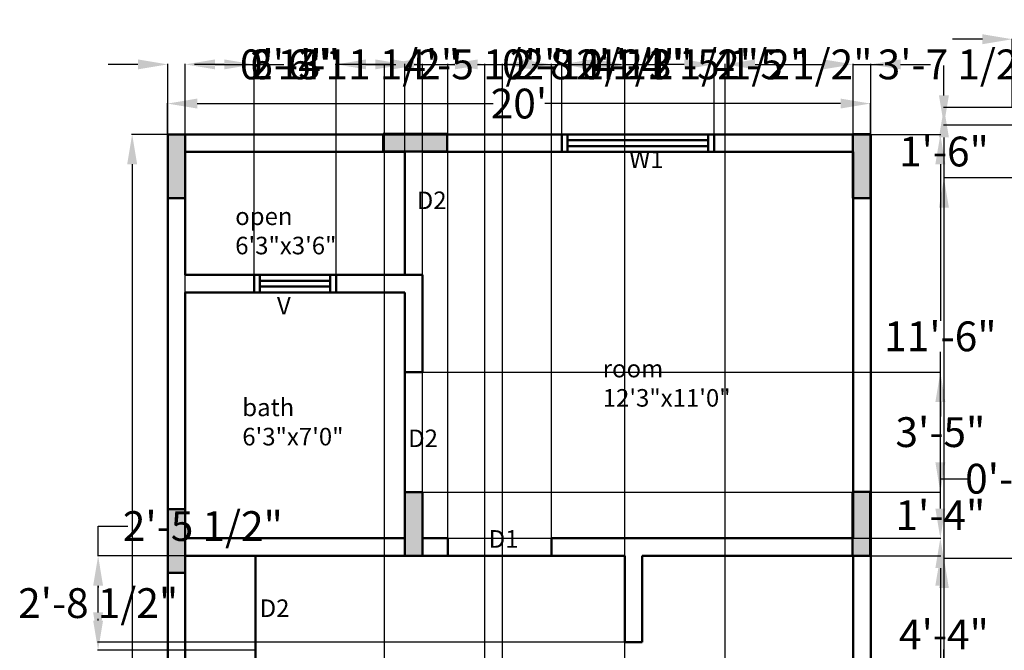
# Model space of a CAD drawing. Units: inches. Extents: x 21 to 3450, y 4 to 2137.
# Tile 2 of 14: x 2177 to 2513, y 1321 to 1537. Entities that reach past the tile are written whole.
import ezdxf

# ---------------------------------------------------------------- set-up
doc = ezdxf.new("R2010")
doc.units = ezdxf.units.IN
doc.header["$MEASUREMENT"] = 0
for name, color, linetype, lineweight in [('A-ANNO-DIMS', 2, 'Continuous', 18), ('A-ANNO-TEXT', 7, 'Continuous', 18), ('A-AREA-IDEN', 3, 'Continuous', 18), ('A-WALL', 7, 'Continuous', 50), ('A-WALL-PATT', 8, 'Continuous', 13)]:
    doc.layers.add(name, color=color, linetype=linetype, lineweight=lineweight)
doc.styles.get("Standard").update_dxf_attribs({"font": 'arial.ttf'})
doc.dimstyles.get("Standard").update_dxf_attribs({"dimtxt": 10.18, "dimasz": 10.18, "dimexe": 0.18, "dimexo": 0.0625, "dimgap": 0.09, "dimtad": 0, "dimtih": 1, "dimtoh": 1, "dimdec": 0, "dimzin": 0, "dimdsep": 46, "dimlunit": 3, "dimtxsty": 'Standard', "dimcen": 0.09, "dimadec": 0, "dimazin": 0, "dimtfac": 1, "dimtdec": 0, "dimtofl": 0, "dimtmove": 0, "dimatfit": 3, "dimfxl": 1, "dimtolj": 1, "dimtzin": 0, "dimarcsym": 0})

# ---------------------------------------------------------------- blocks, each defined once
blk = doc.blocks.new('*D1')
at = {"layer": 'A-ANNO-DIMS', "color": 0, "lineweight": -2, "transparency": 16777216}
for p, q in [((2227.33, 1497.5), (2215.09, 1497.5)), ((2215.27, 1487.32), (2215.27, 1292.79)), ((2215.27, 1087.68), (2215.27, 1282.21)), ((2227.33, 1077.5), (2215.09, 1077.5))]:
    blk.add_line(p, q, dxfattribs=at)
at = {"layer": 'A-ANNO-DIMS', "color": 0, "transparency": 16777216}
for points in [[(2213.57, 1487.32), (2216.97, 1487.32), (2215.27, 1497.5)], [(2213.57, 1087.68), (2216.97, 1087.68), (2215.27, 1077.5)]]:
    blk.add_solid(points, dxfattribs=at)
at = {"layer": 'Defpoints', "color": 0, "transparency": 16777216}
for p in [(2227.4, 1497.5), (2215.27, 1077.5), (2227.4, 1077.5)]:
    blk.add_point(p, dxfattribs=at)
at = {"layer": 'A-ANNO-DIMS', "color": 0, "transparency": 16777216, "insert": (2215.27, 1287.5), "char_height": 10.18, "attachment_point": 5}
blk.add_mtext("\\A1;35'", dxfattribs=at)
blk = doc.blocks.new('*D2')
at = {"layer": 'A-ANNO-DIMS', "color": 0, "lineweight": -2, "transparency": 16777216}
for p, q in [((2227.33, 1497.56), (2227.33, 1508.21)), ((2237.51, 1508.03), (2338.48, 1508.03)), ((2457.08, 1508.03), (2356.11, 1508.03)), ((2467.26, 1497.56), (2467.26, 1508.21))]:
    blk.add_line(p, q, dxfattribs=at)
at = {"layer": 'A-ANNO-DIMS', "color": 0, "transparency": 16777216}
for points in [[(2237.51, 1509.73), (2237.51, 1506.33), (2227.33, 1508.03)], [(2457.08, 1509.73), (2457.08, 1506.33), (2467.26, 1508.03)]]:
    blk.add_solid(points, dxfattribs=at)
at = {"layer": 'Defpoints', "color": 0, "transparency": 16777216}
for p in [(2467.26, 1508.03), (2227.33, 1497.5), (2467.26, 1497.5)]:
    blk.add_point(p, dxfattribs=at)
at = {"layer": 'A-ANNO-DIMS', "color": 0, "transparency": 16777216, "insert": (2347.3, 1508.03), "char_height": 10.18, "attachment_point": 5}
blk.add_mtext("\\A1;20'", dxfattribs=at)
blk = doc.blocks.new('*D34')
at = {"layer": 'A-ANNO-DIMS', "color": 0, "lineweight": -2, "transparency": 16777216}
for p, q in [((2217.22, 1521.41), (2207.04, 1521.41)), ((2227.4, 1497.56), (2227.4, 1521.59)), ((2233.4, 1491.56), (2233.4, 1521.59)), ((2243.58, 1521.41), (2253.76, 1521.41))]:
    blk.add_line(p, q, dxfattribs=at)
at = {"layer": 'A-ANNO-DIMS', "color": 0, "transparency": 16777216}
for points in [[(2217.22, 1523.11), (2217.22, 1519.72), (2227.4, 1521.41)], [(2243.58, 1523.11), (2243.58, 1519.72), (2233.4, 1521.41)]]:
    blk.add_solid(points, dxfattribs=at)
at = {"layer": 'Defpoints', "color": 0, "transparency": 16777216}
for p in [(2233.4, 1521.41), (2227.4, 1497.5), (2233.4, 1491.5)]:
    blk.add_point(p, dxfattribs=at)
at = {"layer": 'A-ANNO-DIMS', "color": 0, "transparency": 16777216, "insert": (2267.38, 1521.41), "char_height": 10.18, "attachment_point": 5}
blk.add_mtext('\\A1;0\'-6"', dxfattribs=at)
blk = doc.blocks.new('*D35')
at = {"layer": 'A-ANNO-DIMS', "color": 0, "lineweight": -2, "transparency": 16777216}
for p, q in [((2233.4, 1491.56), (2233.4, 1521.59)), ((2243.58, 1521.41), (2257.25, 1521.41)), ((2298.22, 1521.41), (2284.54, 1521.41)), ((2308.4, 1491.56), (2308.4, 1521.59))]:
    blk.add_line(p, q, dxfattribs=at)
at = {"layer": 'A-ANNO-DIMS', "color": 0, "transparency": 16777216}
for points in [[(2243.58, 1523.11), (2243.58, 1519.72), (2233.4, 1521.41)], [(2298.22, 1523.11), (2298.22, 1519.72), (2308.4, 1521.41)]]:
    blk.add_solid(points, dxfattribs=at)
at = {"layer": 'Defpoints', "color": 0, "transparency": 16777216}
for p in [(2308.4, 1521.41), (2233.4, 1491.5), (2308.4, 1491.5)]:
    blk.add_point(p, dxfattribs=at)
at = {"layer": 'A-ANNO-DIMS', "color": 0, "transparency": 16777216, "insert": (2270.9, 1521.41), "char_height": 10.18, "attachment_point": 5}
blk.add_mtext('\\A1;6\'-3"', dxfattribs=at)
blk = doc.blocks.new('*D36')
at = {"layer": 'A-ANNO-DIMS', "color": 0, "lineweight": -2, "transparency": 16777216}
for p, q in [((2298.22, 1521.41), (2288.04, 1521.41)), ((2308.4, 1491.56), (2308.4, 1521.59)), ((2361.9, 1497.56), (2361.9, 1521.59)), ((2372.08, 1521.41), (2382.26, 1521.41))]:
    blk.add_line(p, q, dxfattribs=at)
at = {"layer": 'A-ANNO-DIMS', "color": 0, "transparency": 16777216}
for points in [[(2298.22, 1523.11), (2298.22, 1519.72), (2308.4, 1521.41)], [(2372.08, 1523.11), (2372.08, 1519.72), (2361.9, 1521.41)]]:
    blk.add_solid(points, dxfattribs=at)
at = {"layer": 'Defpoints', "color": 0, "transparency": 16777216}
for p in [(2361.9, 1521.41), (2361.9, 1497.5), (2308.4, 1491.5)]:
    blk.add_point(p, dxfattribs=at)
at = {"layer": 'A-ANNO-DIMS', "color": 0, "transparency": 16777216, "insert": (2335.15, 1521.41), "char_height": 10.18, "attachment_point": 5}
blk.add_mtext('\\A1;4\'-5 1/2"', dxfattribs=at)
blk = doc.blocks.new('*D37')
at = {"layer": 'A-ANNO-DIMS', "color": 0, "lineweight": -2, "transparency": 16777216}
for p, q in [((2361.9, 1497.56), (2361.9, 1521.59)), ((2372.08, 1521.41), (2374.07, 1521.41)), ((2403.72, 1521.41), (2401.72, 1521.41)), ((2413.9, 1497.56), (2413.9, 1521.59))]:
    blk.add_line(p, q, dxfattribs=at)
at = {"layer": 'A-ANNO-DIMS', "color": 0, "transparency": 16777216}
for points in [[(2372.08, 1523.11), (2372.08, 1519.72), (2361.9, 1521.41)], [(2403.72, 1523.11), (2403.72, 1519.72), (2413.9, 1521.41)]]:
    blk.add_solid(points, dxfattribs=at)
at = {"layer": 'Defpoints', "color": 0, "transparency": 16777216}
for p in [(2413.9, 1521.41), (2361.9, 1497.5), (2413.9, 1497.5)]:
    blk.add_point(p, dxfattribs=at)
at = {"layer": 'A-ANNO-DIMS', "color": 0, "transparency": 16777216, "insert": (2387.9, 1521.41), "char_height": 10.18, "attachment_point": 5}
blk.add_mtext('\\A1;4\'-4"', dxfattribs=at)
blk = doc.blocks.new('*D38')
at = {"layer": 'A-ANNO-DIMS', "color": 0, "lineweight": -2, "transparency": 16777216}
for p, q in [((2403.72, 1521.41), (2393.54, 1521.41)), ((2413.9, 1497.56), (2413.9, 1521.59)), ((2467.4, 1497.56), (2467.4, 1521.59)), ((2477.58, 1521.41), (2487.76, 1521.41))]:
    blk.add_line(p, q, dxfattribs=at)
at = {"layer": 'A-ANNO-DIMS', "color": 0, "transparency": 16777216}
for points in [[(2403.72, 1523.11), (2403.72, 1519.72), (2413.9, 1521.41)], [(2477.58, 1523.11), (2477.58, 1519.72), (2467.4, 1521.41)]]:
    blk.add_solid(points, dxfattribs=at)
at = {"layer": 'Defpoints', "color": 0, "transparency": 16777216}
for p in [(2467.4, 1521.41), (2413.9, 1497.5), (2467.4, 1497.5)]:
    blk.add_point(p, dxfattribs=at)
at = {"layer": 'A-ANNO-DIMS', "color": 0, "transparency": 16777216, "insert": (2440.65, 1521.41), "char_height": 10.18, "attachment_point": 5}
blk.add_mtext('\\A1;4\'-5 1/2"', dxfattribs=at)
blk = doc.blocks.new('*D47')
at = {"layer": 'A-ANNO-DIMS', "color": 0, "lineweight": -2, "transparency": 16777216}
for p, q in [((2461.25, 1353.55), (2491.33, 1353.55)), ((2491.15, 1343.37), (2491.15, 1298.81)), ((2491.15, 1243.68), (2491.15, 1288.24)), ((2461.46, 1233.5), (2491.33, 1233.5))]:
    blk.add_line(p, q, dxfattribs=at)
at = {"layer": 'A-ANNO-DIMS', "color": 0, "transparency": 16777216}
for points in [[(2489.45, 1343.37), (2492.84, 1343.37), (2491.15, 1353.55)], [(2489.45, 1243.68), (2492.84, 1243.68), (2491.15, 1233.5)]]:
    blk.add_solid(points, dxfattribs=at)
at = {"layer": 'Defpoints', "color": 0, "transparency": 16777216}
for p in [(2461.19, 1353.55), (2491.15, 1353.55), (2461.4, 1233.5)]:
    blk.add_point(p, dxfattribs=at)
at = {"layer": 'A-ANNO-DIMS', "color": 0, "transparency": 16777216, "insert": (2491.15, 1293.53), "char_height": 10.18, "attachment_point": 5}
blk.add_mtext('\\A1;10\'-0"', dxfattribs=at)
blk = doc.blocks.new('*D48')
at = {"layer": 'A-ANNO-DIMS', "color": 0, "lineweight": -2, "transparency": 16777216}
for p, q in [((2491.15, 1369.68), (2491.15, 1379.86)), ((2491.15, 1379.86), (2501.33, 1379.86)), ((2461.46, 1359.5), (2491.33, 1359.5)), ((2461.25, 1353.55), (2491.33, 1353.55)), ((2491.15, 1343.37), (2491.15, 1333.19))]:
    blk.add_line(p, q, dxfattribs=at)
at = {"layer": 'A-ANNO-DIMS', "color": 0, "transparency": 16777216}
for points in [[(2489.45, 1369.68), (2492.84, 1369.68), (2491.15, 1359.5)], [(2489.45, 1343.37), (2492.84, 1343.37), (2491.15, 1353.55)]]:
    blk.add_solid(points, dxfattribs=at)
at = {"layer": 'Defpoints', "color": 0, "transparency": 16777216}
for p in [(2461.4, 1359.5), (2491.15, 1359.5), (2461.19, 1353.55)]:
    blk.add_point(p, dxfattribs=at)
at = {"layer": 'A-ANNO-DIMS', "color": 0, "transparency": 16777216, "insert": (2514.95, 1379.86), "char_height": 10.18, "attachment_point": 5}
blk.add_mtext('\\A1;0\'-6"', dxfattribs=at)
blk = doc.blocks.new('*D49')
at = {"layer": 'A-ANNO-DIMS', "color": 0, "lineweight": -2, "transparency": 16777216}
for p, q in [((2467.46, 1497.5), (2491.33, 1497.5)), ((2491.15, 1487.32), (2491.15, 1433.78)), ((2491.15, 1369.68), (2491.15, 1423.21)), ((2461.46, 1359.5), (2491.33, 1359.5))]:
    blk.add_line(p, q, dxfattribs=at)
at = {"layer": 'A-ANNO-DIMS', "color": 0, "transparency": 16777216}
for points in [[(2489.45, 1487.32), (2492.84, 1487.32), (2491.15, 1497.5)], [(2489.45, 1369.68), (2492.84, 1369.68), (2491.15, 1359.5)]]:
    blk.add_solid(points, dxfattribs=at)
at = {"layer": 'Defpoints', "color": 0, "transparency": 16777216}
for p in [(2467.4, 1497.5), (2491.15, 1497.5), (2461.4, 1359.5)]:
    blk.add_point(p, dxfattribs=at)
at = {"layer": 'A-ANNO-DIMS', "color": 0, "transparency": 16777216, "insert": (2491.15, 1428.5), "char_height": 10.18, "attachment_point": 5}
blk.add_mtext('\\A1;11\'-6"', dxfattribs=at)
blk = doc.blocks.new('*D50')
at = {"layer": 'A-ANNO-DIMS', "color": 0, "lineweight": -2, "transparency": 16777216}
for p, q in [((2203.65, 1353.5), (2203.65, 1363.68)), ((2203.65, 1363.68), (2213.83, 1363.68)), ((2383.33, 1353.5), (2203.47, 1353.5)), ((2203.65, 1334.19), (2203.65, 1343.32)), ((2383.33, 1324.01), (2203.47, 1324.01))]:
    blk.add_line(p, q, dxfattribs=at)
at = {"layer": 'A-ANNO-DIMS', "color": 0, "transparency": 16777216}
for points in [[(2201.95, 1343.32), (2205.34, 1343.32), (2203.65, 1353.5)], [(2201.95, 1334.19), (2205.34, 1334.19), (2203.65, 1324.01)]]:
    blk.add_solid(points, dxfattribs=at)
at = {"layer": 'Defpoints', "color": 0, "transparency": 16777216}
for p in [(2203.65, 1353.5), (2383.4, 1353.5), (2383.4, 1324.01)]:
    blk.add_point(p, dxfattribs=at)
at = {"layer": 'A-ANNO-DIMS', "color": 0, "transparency": 16777216, "insert": (2239.39, 1363.68), "char_height": 10.18, "attachment_point": 5}
blk.add_mtext('\\A1;2\'-5 1/2"', dxfattribs=at)
blk = doc.blocks.new('*D52')
at = {"layer": 'A-ANNO-DIMS', "color": 0, "lineweight": -2, "transparency": 16777216}
for p, q in [((2323.02, 1353.56), (2323.02, 1521.59)), ((2333.2, 1521.41), (2348.18, 1521.41)), ((2358.36, 1353.56), (2358.36, 1521.59)), ((2358.36, 1521.41), (2368.54, 1521.41))]:
    blk.add_line(p, q, dxfattribs=at)
at = {"layer": 'A-ANNO-DIMS', "color": 0, "transparency": 16777216}
for points in [[(2333.2, 1523.11), (2333.2, 1519.72), (2323.02, 1521.41)], [(2348.18, 1523.11), (2348.18, 1519.72), (2358.36, 1521.41)]]:
    blk.add_solid(points, dxfattribs=at)
at = {"layer": 'Defpoints', "color": 0, "transparency": 16777216}
for p in [(2358.36, 1521.41), (2323.02, 1353.5), (2358.36, 1353.5)]:
    blk.add_point(p, dxfattribs=at)
at = {"layer": 'A-ANNO-DIMS', "color": 0, "transparency": 16777216, "insert": (2398.06, 1521.41), "char_height": 10.18, "attachment_point": 5}
blk.add_mtext('\\A1;2\'-11 1/2"', dxfattribs=at)
blk = doc.blocks.new('*D53')
at = {"layer": 'A-ANNO-DIMS', "color": 0, "lineweight": -2, "transparency": 16777216}
for p, q in [((2304.19, 1521.41), (2294.01, 1521.41)), ((2314.37, 1353.56), (2314.37, 1521.59)), ((2323.02, 1353.56), (2323.02, 1521.59)), ((2333.2, 1521.41), (2343.38, 1521.41))]:
    blk.add_line(p, q, dxfattribs=at)
at = {"layer": 'A-ANNO-DIMS', "color": 0, "transparency": 16777216}
for points in [[(2304.19, 1523.11), (2304.19, 1519.72), (2314.37, 1521.41)], [(2333.2, 1523.11), (2333.2, 1519.72), (2323.02, 1521.41)]]:
    blk.add_solid(points, dxfattribs=at)
at = {"layer": 'Defpoints', "color": 0, "transparency": 16777216}
for p in [(2323.02, 1521.41), (2314.37, 1353.5), (2323.02, 1353.5)]:
    blk.add_point(p, dxfattribs=at)
at = {"layer": 'A-ANNO-DIMS', "color": 0, "transparency": 16777216, "insert": (2368.86, 1521.41), "char_height": 10.18, "attachment_point": 5}
blk.add_mtext('\\A1;0\'-8 1/2"', dxfattribs=at)
blk = doc.blocks.new('*D54')
at = {"layer": 'A-ANNO-DIMS', "color": 0, "lineweight": -2, "transparency": 16777216}
for p, q in [((2314.46, 1416.26), (2491.33, 1416.26)), ((2491.15, 1406.08), (2491.15, 1401.06)), ((2491.15, 1385.46), (2491.15, 1390.48)), ((2314.43, 1375.28), (2491.33, 1375.28))]:
    blk.add_line(p, q, dxfattribs=at)
at = {"layer": 'A-ANNO-DIMS', "color": 0, "transparency": 16777216}
for points in [[(2489.45, 1406.08), (2492.84, 1406.08), (2491.15, 1416.26)], [(2489.45, 1385.46), (2492.84, 1385.46), (2491.15, 1375.28)]]:
    blk.add_solid(points, dxfattribs=at)
at = {"layer": 'Defpoints', "color": 0, "transparency": 16777216}
for p in [(2314.4, 1416.26), (2491.15, 1416.26), (2314.37, 1375.28)]:
    blk.add_point(p, dxfattribs=at)
at = {"layer": 'A-ANNO-DIMS', "color": 0, "transparency": 16777216, "insert": (2491.15, 1395.77), "char_height": 10.18, "attachment_point": 5}
blk.add_mtext('\\A1;3\'-5"', dxfattribs=at)
blk = doc.blocks.new('*D55')
at = {"layer": 'A-ANNO-DIMS', "color": 0, "lineweight": -2, "transparency": 16777216}
for p, q in [((2491.15, 1385.46), (2491.15, 1395.64)), ((2314.43, 1375.28), (2491.33, 1375.28)), ((2314.46, 1359.5), (2491.33, 1359.5)), ((2491.15, 1349.32), (2491.15, 1339.14))]:
    blk.add_line(p, q, dxfattribs=at)
at = {"layer": 'A-ANNO-DIMS', "color": 0, "transparency": 16777216}
for points in [[(2489.45, 1385.46), (2492.84, 1385.46), (2491.15, 1375.28)], [(2489.45, 1349.32), (2492.84, 1349.32), (2491.15, 1359.5)]]:
    blk.add_solid(points, dxfattribs=at)
at = {"layer": 'Defpoints', "color": 0, "transparency": 16777216}
for p in [(2314.37, 1375.28), (2491.15, 1375.28), (2314.4, 1359.5)]:
    blk.add_point(p, dxfattribs=at)
at = {"layer": 'A-ANNO-DIMS', "color": 0, "transparency": 16777216, "insert": (2491.15, 1367.39), "char_height": 10.18, "attachment_point": 5}
blk.add_mtext('\\A1;1\'-4"', dxfattribs=at)
blk = doc.blocks.new('*D56')
at = {"layer": 'A-ANNO-DIMS', "color": 0, "lineweight": -2, "transparency": 16777216}
for p, q in [((2257.33, 1353.5), (2203.47, 1353.5)), ((2203.65, 1343.32), (2203.65, 1342.72)), ((2203.65, 1331.41), (2203.65, 1332.01)), ((2257.33, 1321.23), (2203.47, 1321.23))]:
    blk.add_line(p, q, dxfattribs=at)
at = {"layer": 'A-ANNO-DIMS', "color": 0, "transparency": 16777216}
for points in [[(2201.95, 1343.32), (2205.34, 1343.32), (2203.65, 1353.5)], [(2201.95, 1331.41), (2205.34, 1331.41), (2203.65, 1321.23)]]:
    blk.add_solid(points, dxfattribs=at)
at = {"layer": 'Defpoints', "color": 0, "transparency": 16777216}
for p in [(2203.65, 1353.5), (2257.4, 1353.5), (2257.4, 1321.23)]:
    blk.add_point(p, dxfattribs=at)
at = {"layer": 'A-ANNO-DIMS', "color": 0, "transparency": 16777216, "insert": (2203.65, 1337.36), "char_height": 10.18, "attachment_point": 5}
blk.add_mtext('\\A1;2\'-8 1/2"', dxfattribs=at)
blk = doc.blocks.new('*D57')
at = {"layer": 'A-ANNO-DIMS', "color": 0, "lineweight": -2, "transparency": 16777216}
for p, q in [((2301.35, 1233.56), (2301.35, 1521.59)), ((2311.53, 1521.41), (2325.47, 1521.41)), ((2335.65, 1233.56), (2335.65, 1521.59)), ((2335.65, 1521.41), (2345.83, 1521.41))]:
    blk.add_line(p, q, dxfattribs=at)
at = {"layer": 'A-ANNO-DIMS', "color": 0, "transparency": 16777216}
for points in [[(2311.53, 1523.11), (2311.53, 1519.72), (2301.35, 1521.41)], [(2325.47, 1523.11), (2325.47, 1519.72), (2335.65, 1521.41)]]:
    blk.add_solid(points, dxfattribs=at)
at = {"layer": 'Defpoints', "color": 0, "transparency": 16777216}
for p in [(2335.65, 1521.41), (2301.35, 1233.5), (2335.65, 1233.5)]:
    blk.add_point(p, dxfattribs=at)
at = {"layer": 'A-ANNO-DIMS', "color": 0, "transparency": 16777216, "insert": (2375.36, 1521.41), "char_height": 10.18, "attachment_point": 5}
blk.add_mtext('\\A1;2\'-10 1/2"', dxfattribs=at)
blk = doc.blocks.new('*D58')
at = {"layer": 'A-ANNO-DIMS', "color": 0, "lineweight": -2, "transparency": 16777216}
for p, q in [((2341.65, 1233.56), (2341.65, 1521.59)), ((2351.83, 1521.41), (2373.22, 1521.41)), ((2383.4, 1233.56), (2383.4, 1521.59)), ((2383.4, 1521.41), (2393.58, 1521.41))]:
    blk.add_line(p, q, dxfattribs=at)
at = {"layer": 'A-ANNO-DIMS', "color": 0, "transparency": 16777216}
for points in [[(2351.83, 1523.11), (2351.83, 1519.72), (2341.65, 1521.41)], [(2373.22, 1523.11), (2373.22, 1519.72), (2383.4, 1521.41)]]:
    blk.add_solid(points, dxfattribs=at)
at = {"layer": 'Defpoints', "color": 0, "transparency": 16777216}
for p in [(2383.4, 1521.41), (2341.65, 1233.5), (2383.4, 1233.5)]:
    blk.add_point(p, dxfattribs=at)
at = {"layer": 'A-ANNO-DIMS', "color": 0, "transparency": 16777216, "insert": (2419.05, 1521.41), "char_height": 10.18, "attachment_point": 5}
blk.add_mtext('\\A1;3\'-5 1/2"', dxfattribs=at)
blk = doc.blocks.new('*D61')
at = {"layer": 'A-ANNO-DIMS', "color": 0, "lineweight": -2, "transparency": 16777216}
for p, q in [((2233.4, 1443.56), (2233.4, 1521.59)), ((2243.58, 1521.41), (2246.72, 1521.41)), ((2256.9, 1443.56), (2256.9, 1521.59)), ((2256.9, 1521.41), (2267.08, 1521.41))]:
    blk.add_line(p, q, dxfattribs=at)
at = {"layer": 'A-ANNO-DIMS', "color": 0, "transparency": 16777216}
for points in [[(2243.58, 1523.11), (2243.58, 1519.72), (2233.4, 1521.41)], [(2246.72, 1523.11), (2246.72, 1519.72), (2256.9, 1521.41)]]:
    blk.add_solid(points, dxfattribs=at)
at = {"layer": 'Defpoints', "color": 0, "transparency": 16777216}
for p in [(2256.9, 1521.41), (2233.4, 1443.5), (2256.9, 1443.5)]:
    blk.add_point(p, dxfattribs=at)
at = {"layer": 'A-ANNO-DIMS', "color": 0, "transparency": 16777216, "insert": (2296.03, 1521.41), "char_height": 10.18, "attachment_point": 5}
blk.add_mtext('\\A1;1\'-11 1/2"', dxfattribs=at)
blk = doc.blocks.new('*D62')
at = {"layer": 'A-ANNO-DIMS', "color": 0, "lineweight": -2, "transparency": 16777216}
for p, q in [((2246.72, 1521.41), (2236.54, 1521.41)), ((2256.9, 1443.56), (2256.9, 1521.59)), ((2284.9, 1443.56), (2284.9, 1521.59)), ((2295.08, 1521.41), (2305.26, 1521.41))]:
    blk.add_line(p, q, dxfattribs=at)
at = {"layer": 'A-ANNO-DIMS', "color": 0, "transparency": 16777216}
for points in [[(2246.72, 1523.11), (2246.72, 1519.72), (2256.9, 1521.41)], [(2295.08, 1523.11), (2295.08, 1519.72), (2284.9, 1521.41)]]:
    blk.add_solid(points, dxfattribs=at)
at = {"layer": 'Defpoints', "color": 0, "transparency": 16777216}
for p in [(2284.9, 1521.41), (2256.9, 1443.5), (2284.9, 1443.5)]:
    blk.add_point(p, dxfattribs=at)
at = {"layer": 'A-ANNO-DIMS', "color": 0, "transparency": 16777216, "insert": (2270.9, 1521.41), "char_height": 10.18, "attachment_point": 5}
blk.add_mtext('\\A1;2\'-4"', dxfattribs=at)
blk = doc.blocks.new('*D63')
at = {"layer": 'A-ANNO-DIMS', "color": 0, "lineweight": -2, "transparency": 16777216}
for p, q in [((2417.71, 1189.56), (2417.71, 1521.59)), ((2427.89, 1521.41), (2451.22, 1521.41)), ((2461.4, 1189.56), (2461.4, 1521.59)), ((2461.4, 1521.41), (2471.58, 1521.41))]:
    blk.add_line(p, q, dxfattribs=at)
at = {"layer": 'A-ANNO-DIMS', "color": 0, "transparency": 16777216}
for points in [[(2427.89, 1523.11), (2427.89, 1519.72), (2417.71, 1521.41)], [(2451.22, 1523.11), (2451.22, 1519.72), (2461.4, 1521.41)]]:
    blk.add_solid(points, dxfattribs=at)
at = {"layer": 'Defpoints', "color": 0, "transparency": 16777216}
for p in [(2461.4, 1521.41), (2417.71, 1189.5), (2461.4, 1189.5)]:
    blk.add_point(p, dxfattribs=at)
at = {"layer": 'A-ANNO-DIMS', "color": 0, "transparency": 16777216, "insert": (2497.05, 1521.41), "char_height": 10.18, "attachment_point": 5}
blk.add_mtext('\\A1;3\'-7 1/2"', dxfattribs=at)
blk = doc.blocks.new('*D67')
at = {"layer": 'A-ANNO-DIMS', "color": 0, "lineweight": -2, "transparency": 16777216}
for p, q in [((2515.64, 1506.65), (2492.19, 1506.65)), ((2492.37, 1496.47), (2492.37, 1301.94)), ((2492.37, 1096.83), (2492.37, 1291.36)), ((2515.56, 1086.65), (2492.19, 1086.65))]:
    blk.add_line(p, q, dxfattribs=at)
at = {"layer": 'A-ANNO-DIMS', "color": 0, "transparency": 16777216}
for points in [[(2490.67, 1496.47), (2494.06, 1496.47), (2492.37, 1506.65)], [(2490.67, 1096.83), (2494.06, 1096.83), (2492.37, 1086.65)]]:
    blk.add_solid(points, dxfattribs=at)
at = {"layer": 'Defpoints', "color": 0, "transparency": 16777216}
for p in [(2492.37, 1506.65), (2515.71, 1506.65), (2515.62, 1086.65)]:
    blk.add_point(p, dxfattribs=at)
at = {"layer": 'A-ANNO-DIMS', "color": 0, "transparency": 16777216, "insert": (2492.37, 1296.65), "char_height": 10.18, "attachment_point": 5}
blk.add_mtext('\\A1;35\'-0"', dxfattribs=at)
blk = doc.blocks.new('*D68')
at = {"layer": 'A-ANNO-DIMS', "color": 0, "lineweight": -2, "transparency": 16777216}
for p, q in [((2505.53, 1530.01), (2495.35, 1530.01)), ((2515.71, 1506.71), (2515.71, 1530.19)), ((2521.71, 1500.71), (2521.71, 1530.19)), ((2531.89, 1530.01), (2542.07, 1530.01))]:
    blk.add_line(p, q, dxfattribs=at)
at = {"layer": 'A-ANNO-DIMS', "color": 0, "transparency": 16777216}
for points in [[(2505.53, 1531.71), (2505.53, 1528.31), (2515.71, 1530.01)], [(2531.89, 1531.71), (2531.89, 1528.31), (2521.71, 1530.01)]]:
    blk.add_solid(points, dxfattribs=at)
at = {"layer": 'Defpoints', "color": 0, "transparency": 16777216}
for p in [(2521.71, 1530.01), (2515.71, 1506.65), (2521.71, 1500.65)]:
    blk.add_point(p, dxfattribs=at)
at = {"layer": 'A-ANNO-DIMS', "color": 0, "transparency": 16777216, "insert": (2555.69, 1530.01), "char_height": 10.18, "attachment_point": 5}
blk.add_mtext('\\A1;0\'-6"', dxfattribs=at)
blk = doc.blocks.new('*D81')
at = {"layer": 'A-ANNO-DIMS', "color": 0, "lineweight": -2, "transparency": 16777216}
for p, q in [((2492.37, 1510.83), (2492.37, 1521.01)), ((2521.64, 1500.65), (2492.19, 1500.65)), ((2521.64, 1482.65), (2492.19, 1482.65)), ((2492.37, 1472.47), (2492.37, 1462.29))]:
    blk.add_line(p, q, dxfattribs=at)
at = {"layer": 'A-ANNO-DIMS', "color": 0, "transparency": 16777216}
for points in [[(2490.67, 1510.83), (2494.06, 1510.83), (2492.37, 1500.65)], [(2490.67, 1472.47), (2494.06, 1472.47), (2492.37, 1482.65)]]:
    blk.add_solid(points, dxfattribs=at)
at = {"layer": 'Defpoints', "color": 0, "transparency": 16777216}
for p in [(2492.37, 1500.65), (2521.71, 1500.65), (2521.71, 1482.65)]:
    blk.add_point(p, dxfattribs=at)
at = {"layer": 'A-ANNO-DIMS', "color": 0, "transparency": 16777216, "insert": (2492.37, 1491.65), "char_height": 10.18, "attachment_point": 5}
blk.add_mtext('\\A1;1\'-6"', dxfattribs=at)
blk = doc.blocks.new('*D89')
at = {"layer": 'A-ANNO-DIMS', "color": 0, "lineweight": -2, "transparency": 16777216}
for p, q in [((2545.64, 1352.65), (2492.19, 1352.65)), ((2492.37, 1342.47), (2492.37, 1331.83)), ((2492.37, 1310.83), (2492.37, 1321.47)), ((2545.64, 1300.65), (2492.19, 1300.65))]:
    blk.add_line(p, q, dxfattribs=at)
at = {"layer": 'A-ANNO-DIMS', "color": 0, "transparency": 16777216}
for points in [[(2490.67, 1342.47), (2494.06, 1342.47), (2492.37, 1352.65)], [(2490.67, 1310.83), (2494.06, 1310.83), (2492.37, 1300.65)]]:
    blk.add_solid(points, dxfattribs=at)
at = {"layer": 'Defpoints', "color": 0, "transparency": 16777216}
for p in [(2492.37, 1352.65), (2545.71, 1352.65), (2545.71, 1300.65)]:
    blk.add_point(p, dxfattribs=at)
at = {"layer": 'A-ANNO-DIMS', "color": 0, "transparency": 16777216, "insert": (2492.37, 1326.65), "char_height": 10.18, "attachment_point": 5}
blk.add_mtext('\\A1;4\'-4"', dxfattribs=at)

msp = doc.modelspace()

# ---------------------------------------------------------------- hatches: boundary and pattern name
at = {"layer": 'A-WALL-PATT'}
h = msp.add_hatch(color=256, dxfattribs=at)
h.dxf.hatch_style = 1
h.paths.add_polyline_path([(2233.4, 1497.5), (2227.4, 1497.5), (2227.4, 1475.71), (2233.4, 1475.71)])
h.paths.add_polyline_path([(2322.77, 1497.5), (2300.98, 1497.5), (2300.98, 1491.66), (2322.77, 1491.66)])
h.paths.add_polyline_path([(2467.26, 1497.5), (2461.26, 1497.5), (2461.26, 1491.5), (2461.4, 1491.5), (2461.4, 1475.76), (2467.26, 1475.76)])
h.paths.add_polyline_path([(2233.4, 1369.46), (2227.4, 1369.46), (2227.4, 1347.68), (2233.4, 1347.68)])
h.paths.add_polyline_path([(2314.37, 1375.28), (2308.4, 1375.28), (2308.4, 1359.5), (2308.37, 1353.5), (2314.37, 1353.5)])
h.paths.add_polyline_path([(2467.19, 1375.34), (2461.4, 1375.34), (2461.4, 1359.5), (2461.19, 1353.55), (2467.19, 1353.55)])
h.paths.add_polyline_path([(2467.34, 1243.32), (2461.4, 1243.32), (2461.4, 1233.5), (2461.37, 1227.5), (2461.4, 1227.5), (2461.4, 1221.53), (2467.34, 1221.53)])
h.paths.add_polyline_path([(2341.4, 1227.5), (2341.65, 1227.5), (2341.65, 1233.5), (2335.65, 1233.5), (2335.65, 1211.8), (2341.4, 1211.8)])
h.paths.add_polyline_path([(2233.4, 1241.01), (2227.4, 1241.01), (2227.4, 1219.23), (2233.4, 1219.23)])
h.paths.add_polyline_path([(2341.4, 1099.28), (2335.58, 1099.28), (2335.58, 1077.5), (2341.58, 1077.5), (2341.58, 1083.5), (2341.4, 1083.5)])
h.paths.add_polyline_path([(2467.29, 1099.28), (2461.4, 1099.28), (2461.4, 1083.5), (2461.29, 1077.5), (2467.29, 1077.5)])

# ---------------------------------------------------------------- linework, layer by layer
at = {"layer": 'A-WALL'}
for p, q in [((2227.4, 1077.5), (2227.4, 1497.5)), ((2227.4, 1497.5), (2467.4, 1497.5)), ((2361.9, 1491.5), (2361.9, 1497.5)), ((2363.9, 1491.5), (2363.9, 1497.5)), ((2411.9, 1491.5), (2411.9, 1497.5)), ((2413.9, 1491.5), (2413.9, 1497.5)), ((2467.4, 1497.5), (2467.4, 1077.5)), ((2363.9, 1495.5), (2411.9, 1495.5)), ((2363.9, 1493.5), (2411.9, 1493.5)), ((2233.4, 1491.5), (2308.4, 1491.5)), ((2233.4, 1449.5), (2233.4, 1491.5)), ((2308.4, 1449.5), (2308.4, 1491.5)), ((2314.4, 1491.5), (2461.4, 1491.5)), ((2461.4, 1491.5), (2461.4, 1359.5)), ((2233.4, 1449.5), (2308.4, 1449.5)), ((2256.9, 1449.5), (2256.9, 1443.5)), ((2258.9, 1449.5), (2258.9, 1443.5)), ((2282.9, 1449.5), (2282.9, 1443.5)), ((2284.9, 1449.5), (2284.9, 1443.5)), ((2308.4, 1449.5), (2314.4, 1449.5)), ((2314.4, 1416.26), (2314.4, 1449.5)), ((2258.9, 1447.5), (2282.9, 1447.5)), ((2258.9, 1445.5), (2282.9, 1445.5)), ((2233.4, 1443.5), (2308.4, 1443.5)), ((2233.4, 1359.5), (2233.4, 1443.5)), ((2308.4, 1359.5), (2308.4, 1443.5)), ((2308.4, 1416.26), (2314.4, 1416.26)), ((2233.4, 1359.5), (2308.4, 1359.5)), ((2233.4, 1359.5), (2308.4, 1359.5)), ((2314.4, 1359.5), (2323.02, 1359.5)), ((2314.4, 1359.5), (2323.02, 1359.5)), ((2323.02, 1359.5), (2323.02, 1353.5)), ((2358.36, 1359.5), (2358.36, 1353.5)), ((2358.36, 1359.5), (2461.4, 1359.5)), ((2358.36, 1359.5), (2461.4, 1359.5)), ((2233.4, 1353.5), (2257.4, 1353.5)), ((2233.4, 1233.5), (2233.4, 1353.5)), ((2257.4, 1353.5), (2257.4, 1233.5)), ((2263.4, 1353.5), (2257.4, 1353.5)), ((2263.4, 1353.5), (2383.4, 1353.5)), ((2383.4, 1353.5), (2383.4, 1324.01)), ((2389.4, 1353.5), (2389.4, 1324.01)), ((2389.4, 1353.5), (2461.4, 1353.5)), ((2461.4, 1353.5), (2461.4, 1233.5)), ((2389.4, 1324.01), (2383.4, 1324.01))]:
    msp.add_line(p, q, dxfattribs=at)
for points in [[(2227.4, 1497.5), (2233.4, 1497.5), (2233.4, 1475.71), (2227.4, 1475.71)], [(2300.98, 1491.66), (2300.98, 1497.66), (2322.77, 1497.66), (2322.77, 1491.66)], [(2461.26, 1497.54), (2467.26, 1497.54), (2467.26, 1475.76), (2461.26, 1475.76)], [(2308.37, 1375.28), (2314.37, 1375.28), (2314.37, 1353.5), (2308.37, 1353.5)], [(2461.19, 1375.34), (2467.19, 1375.34), (2467.19, 1353.55), (2461.19, 1353.55)], [(2227.4, 1369.46), (2233.4, 1369.46), (2233.4, 1347.68), (2227.4, 1347.68)]]:
    msp.add_lwpolyline(points, close=True, dxfattribs=at)

# ---------------------------------------------------------------- texts
at = {"layer": 'A-ANNO-TEXT', "char_height": 6, "attachment_point": 1}
for s, insert in [('W1', (2384.92, 1491.97)), ('D2', (2312.42, 1477.97)), ('V', (2264.69, 1441.97)), ('D2', (2309.48, 1396.65)), ('D1', (2336.98, 1362.29)), ('D2', (2258.78, 1338.62))]:
    msp.add_mtext_dynamic_manual_height_columns(s, width=23.0829, gutter_width=1, heights=[0], dxfattribs=dict(at, insert=insert))
at = {"layer": 'A-AREA-IDEN', "char_height": 6, "attachment_point": 1}
for s, insert in [('open \\P6\'3"x3\'6"', (2250.44, 1472.52)), ('room \\P12\'3"x11\'0"', (2375.9, 1420.48)), ('bath \\P6\'3"x7\'0"', (2252.86, 1407.24))]:
    msp.add_mtext_dynamic_manual_height_columns(s, width=31.1036, gutter_width=1, heights=[0], dxfattribs=dict(at, insert=insert))

# ---------------------------------------------------------------- dimensions: what is measured, and where the dimension line sits
at = {"layer": 'A-ANNO-DIMS'}
for base, p1, p2, override, picture, middle in [((2256.9, 1521.41), (2233.4, 1443.5), (2256.9, 1443.5), {"dimdec": 1, "dimlfac": 1, "dimrnd": 0, "dimzin": 1, "dimdsep": 46, "dimlunit": 4, "dimfrac": 2}, '*D61', (2296.03, 1521.41)), ((2361.9, 1521.41), (2308.4, 1491.5), (2361.9, 1497.5), {"dimdec": 1, "dimlfac": 1, "dimrnd": 0, "dimzin": 1, "dimdsep": 46, "dimlunit": 4, "dimfrac": 2}, '*D36', (2335.15, 1521.41)), ((2323.0188, 1521.4135), (2314.3654, 1353.4971), (2323.0188, 1353.4971), {"dimdec": 1, "dimlfac": 1, "dimrnd": 0, "dimzin": 1, "dimdsep": 46, "dimlunit": 4, "dimfrac": 2}, '*D53', (2368.8598, 1521.4135)), ((2335.65, 1521.41), (2301.35, 1233.5), (2335.65, 1233.5), {"dimdec": 1, "dimlfac": 1, "dimrnd": 0, "dimzin": 1, "dimdsep": 46, "dimlunit": 4, "dimfrac": 2}, '*D57', (2375.36, 1521.41)), ((2358.36, 1521.41), (2323.02, 1353.5), (2358.36, 1353.5), {"dimdec": 1, "dimlfac": 1, "dimrnd": 0, "dimzin": 1, "dimdsep": 46, "dimlunit": 4, "dimfrac": 2}, '*D52', (2398.06, 1521.41)), ((2383.3966, 1521.4135), (2341.6544, 1233.4971), (2383.3966, 1233.4971), {"dimdec": 1, "dimlfac": 1, "dimrnd": 0, "dimzin": 1, "dimdsep": 46, "dimlunit": 4, "dimfrac": 2}, '*D58', (2419.0541, 1521.4135)), ((2467.4, 1521.41), (2413.9, 1497.5), (2467.4, 1497.5), {"dimdec": 1, "dimlfac": 1, "dimrnd": 0, "dimzin": 1, "dimdsep": 46, "dimlunit": 4, "dimfrac": 2}, '*D38', (2440.65, 1521.41)), ((2461.4, 1521.41), (2417.71, 1189.5), (2461.4, 1189.5), {"dimdec": 1, "dimlfac": 1, "dimrnd": 0, "dimzin": 1, "dimdsep": 46, "dimlunit": 4, "dimfrac": 2}, '*D63', (2497.05, 1521.41)), ((2521.71, 1530.01), (2515.71, 1506.65), (2521.71, 1500.65), {"dimdec": 1, "dimlfac": 1, "dimrnd": 0, "dimzin": 1, "dimdsep": 46, "dimlunit": 4, "dimfrac": 2}, '*D68', (2555.69, 1530.01)), ((2233.4, 1521.41), (2227.4, 1497.5), (2233.4, 1491.5), {"dimdec": 1, "dimlfac": 1, "dimrnd": 0, "dimzin": 1, "dimdsep": 46, "dimlunit": 4, "dimfrac": 2}, '*D34', (2267.38, 1521.41)), ((2308.4, 1521.41), (2233.4, 1491.5), (2308.4, 1491.5), {"dimdec": 1, "dimlfac": 1, "dimrnd": 0, "dimzin": 1, "dimdsep": 46, "dimlunit": 4, "dimfrac": 2}, '*D35', (2270.9, 1521.41)), ((2284.9, 1521.41), (2256.9, 1443.5), (2284.9, 1443.5), {"dimdec": 1, "dimlfac": 1, "dimrnd": 0, "dimzin": 1, "dimdsep": 46, "dimlunit": 4, "dimfrac": 2}, '*D62', (2270.9, 1521.41)), ((2413.9, 1521.41), (2361.9, 1497.5), (2413.9, 1497.5), {"dimdec": 1, "dimlfac": 1, "dimrnd": 0, "dimzin": 1, "dimdsep": 46, "dimlunit": 4, "dimfrac": 2}, '*D37', (2387.9, 1521.41)), ((2467.26, 1508.03), (2227.33, 1497.5), (2467.26, 1497.5), {"dimclrd": 0, "dimclre": 0, "dimclrt": 0}, '*D2', (2347.3, 1508.03))]:
    dim = msp.add_linear_dim(base=base, p1=p1, p2=p2, dimstyle='Standard', override=override, dxfattribs=at)
    dim.commit()
    dim.dimension.update_dxf_attribs({"geometry": picture, "text_midpoint": middle})
for base, p1, p2, override, picture, middle in [((2492.37, 1500.65), (2521.71, 1482.65), (2521.71, 1500.65), {"dimdec": 1, "dimlfac": 1, "dimrnd": 0, "dimzin": 1, "dimdsep": 46, "dimlunit": 4, "dimfrac": 2}, '*D81', (2492.37, 1491.65)), ((2492.37, 1506.65), (2515.62, 1086.65), (2515.71, 1506.65), {"dimdec": 1, "dimlfac": 1, "dimrnd": 0, "dimzin": 1, "dimdsep": 46, "dimlunit": 4, "dimfrac": 2}, '*D67', (2492.37, 1296.65)), ((2215.27, 1077.5), (2227.4, 1497.5), (2227.4, 1077.5), {"dimclrd": 0, "dimclre": 0, "dimclrt": 0}, '*D1', (2215.27, 1287.5)), ((2491.15, 1497.5), (2461.4, 1359.5), (2467.4, 1497.5), {"dimdec": 1, "dimlfac": 1, "dimrnd": 0, "dimzin": 1, "dimdsep": 46, "dimlunit": 4, "dimfrac": 2}, '*D49', (2491.15, 1428.5)), ((2491.15, 1416.26), (2314.37, 1375.28), (2314.4, 1416.26), {"dimdec": 1, "dimlfac": 1, "dimrnd": 0, "dimzin": 1, "dimdsep": 46, "dimlunit": 4, "dimfrac": 2}, '*D54', (2491.15, 1395.77)), ((2491.15, 1375.28), (2314.4, 1359.5), (2314.37, 1375.28), {"dimdec": 1, "dimlfac": 1, "dimrnd": 0, "dimzin": 1, "dimdsep": 46, "dimlunit": 4, "dimfrac": 2}, '*D55', (2491.15, 1367.39)), ((2491.1466, 1359.4971), (2461.1914, 1353.5544), (2461.3966, 1359.4971), {"dimdec": 1, "dimlfac": 1, "dimrnd": 0, "dimzin": 1, "dimdsep": 46, "dimlunit": 4, "dimfrac": 2}, '*D48', (2514.9471, 1379.8571)), ((2203.65, 1353.5), (2383.4, 1324.01), (2383.4, 1353.5), {"dimdec": 1, "dimlfac": 1, "dimrnd": 0, "dimzin": 1, "dimdsep": 46, "dimlunit": 4, "dimfrac": 2}, '*D50', (2239.39, 1363.68)), ((2203.65, 1353.5), (2257.4, 1321.23), (2257.4, 1353.5), {"dimdec": 1, "dimlfac": 1, "dimrnd": 0, "dimzin": 1, "dimdsep": 46, "dimlunit": 4, "dimfrac": 2}, '*D56', (2203.65, 1337.36)), ((2491.1466, 1353.5544), (2461.3966, 1233.4971), (2461.1914, 1353.5544), {"dimdec": 1, "dimlfac": 1, "dimrnd": 0, "dimzin": 1, "dimdsep": 46, "dimlunit": 4, "dimfrac": 2}, '*D47', (2491.1466, 1293.5257)), ((2492.37, 1352.65), (2545.71, 1300.65), (2545.71, 1352.65), {"dimdec": 1, "dimlfac": 1, "dimrnd": 0, "dimzin": 1, "dimdsep": 46, "dimlunit": 4, "dimfrac": 2}, '*D89', (2492.37, 1326.65))]:
    dim = msp.add_linear_dim(base=base, p1=p1, p2=p2, angle=90, dimstyle='Standard', override=override, dxfattribs=at)
    dim.commit()
    dim.dimension.update_dxf_attribs({"geometry": picture, "text_midpoint": middle})

doc.saveas('drawing.dxf')
